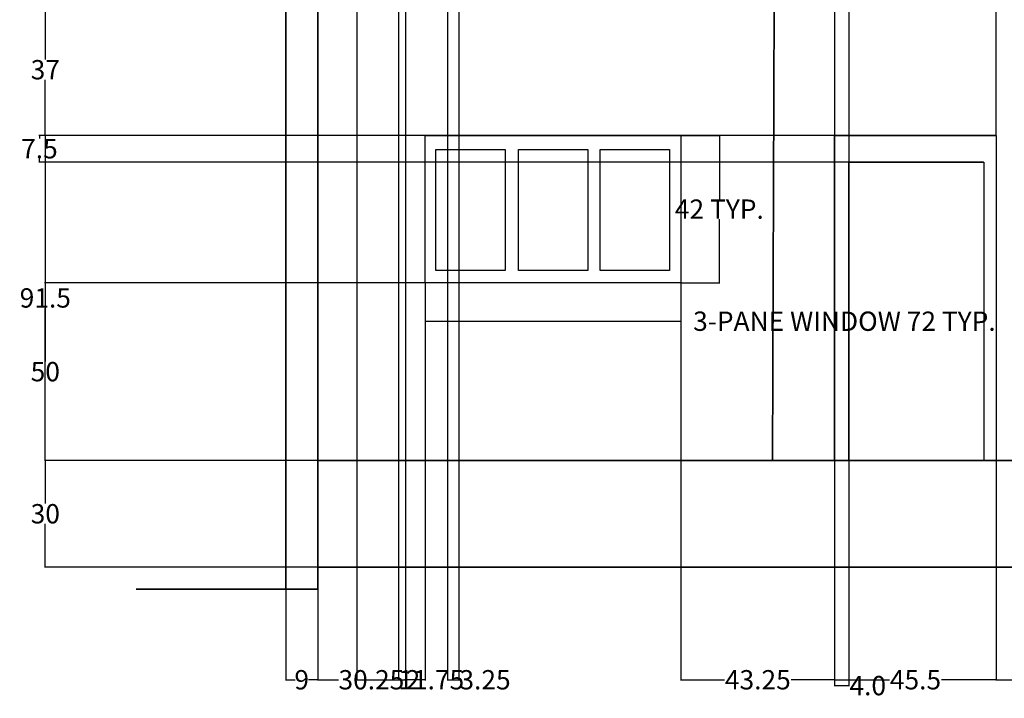
# Model space of a CAD drawing. Units: inches. Extents: x 12 to 590, y 127 to 569.
# Tile 1 of 4: x 17 to 294, y 127 to 318. Entities that reach past the tile are written whole.
import ezdxf

# ---------------------------------------------------------------- set-up
doc = ezdxf.new("R2010")
doc.units = ezdxf.units.IN
doc.header["$MEASUREMENT"] = 0
for name, color, linetype, lineweight in [('A-ANNO-DIMS', 2, 'Continuous', 18), ('A-DOOR', 3, 'Continuous', 25), ('A-ELEV', 7, 'Continuous', 35), ('A-GLAZ', 4, 'Continuous', 25)]:
    doc.layers.add(name, color=color, linetype=linetype, lineweight=lineweight)
doc.styles.get("Standard").update_dxf_attribs({"font": 'arial.ttf'})
doc.dimstyles.get("Standard").update_dxf_attribs({"dimtxt": 5.4375, "dimasz": 0.18, "dimexe": 0.18, "dimexo": 0.0625, "dimgap": 0.09, "dimtad": 0, "dimtih": 1, "dimtoh": 1, "dimdec": 4, "dimzin": 0, "dimdsep": 46, "dimlunit": 4, "dimtxsty": 'Standard', "dimcen": 0.09, "dimadec": 0, "dimazin": 0, "dimtfac": 1, "dimtdec": 4, "dimtofl": 0, "dimtmove": 0, "dimatfit": 3, "dimfxl": 1, "dimtolj": 1, "dimtzin": 0, "dimarcsym": 0})

# ---------------------------------------------------------------- blocks, each defined once
blk = doc.blocks.new('WIN-3PANE')
for points in [[(0, 41.5), (72, 41.5), (72, 0), (0, 0)], [(3, 37.5), (22.5, 37.5), (22.5, 3.5), (3, 3.5)], [(26.25, 37.5), (45.75, 37.5), (45.75, 3.5), (26.25, 3.5)], [(49.25, 37.5), (68.75, 37.5), (68.75, 3.5), (49.25, 3.5)]]:
    blk.add_lwpolyline(points, close=True)
blk = doc.blocks.new('*D3')
at = {"layer": 'A-ANNO-DIMS', "color": 0, "lineweight": -2, "transparency": 16777216}
for p, q in [((130.75, 243.44), (130.75, 232.52)), ((202.75, 243.44), (202.75, 232.52)), ((130.93, 232.7), (202.57, 232.7)), ((202.75, 232.7), (202.93, 232.7))]:
    blk.add_line(p, q, dxfattribs=at)
at = {"layer": 'A-ANNO-DIMS', "color": 0, "transparency": 16777216}
for points in [[(130.93, 232.73), (130.93, 232.67), (130.75, 232.7)], [(202.57, 232.73), (202.57, 232.67), (202.75, 232.7)]]:
    blk.add_solid(points, dxfattribs=at)
at = {"layer": 'Defpoints', "color": 0, "transparency": 16777216}
for p in [(130.75, 243.5), (202.75, 243.5), (202.75, 232.7)]:
    blk.add_point(p, dxfattribs=at)
at = {"layer": 'A-ANNO-DIMS', "color": 0, "transparency": 16777216, "insert": (248.75, 232.7), "char_height": 5.4375, "attachment_point": 5}
blk.add_mtext('\\A1;3-PANE WINDOW 72 TYP.', dxfattribs=at)
blk = doc.blocks.new('*D4')
at = {"layer": 'A-ANNO-DIMS', "color": 0, "lineweight": -2, "transparency": 16777216}
for p, q in [((202.81, 285), (213.73, 285)), ((213.55, 284.82), (213.55, 267.07)), ((213.55, 243.68), (213.55, 261.43)), ((202.81, 243.5), (213.73, 243.5))]:
    blk.add_line(p, q, dxfattribs=at)
at = {"layer": 'A-ANNO-DIMS', "color": 0, "transparency": 16777216}
for points in [[(213.52, 284.82), (213.58, 284.82), (213.55, 285)], [(213.52, 243.68), (213.58, 243.68), (213.55, 243.5)]]:
    blk.add_solid(points, dxfattribs=at)
at = {"layer": 'Defpoints', "color": 0, "transparency": 16777216}
for p in [(202.75, 285), (213.55, 285), (202.75, 243.5)]:
    blk.add_point(p, dxfattribs=at)
at = {"layer": 'A-ANNO-DIMS', "color": 0, "transparency": 16777216, "insert": (213.55, 264.25), "char_height": 5.4375, "attachment_point": 5}
blk.add_mtext('\\A1;42 TYP.', dxfattribs=at)
blk = doc.blocks.new('*D16')
at = {"layer": 'A-ANNO-DIMS', "color": 0, "lineweight": -2, "transparency": 16777216}
for p, q in [((100.44, 193.5), (23.66, 193.5)), ((23.84, 193.32), (23.84, 181.37)), ((23.84, 163.68), (23.84, 175.63)), ((100.44, 163.5), (23.66, 163.5))]:
    blk.add_line(p, q, dxfattribs=at)
at = {"layer": 'A-ANNO-DIMS', "color": 0, "transparency": 16777216}
for points in [[(23.81, 193.32), (23.87, 193.32), (23.84, 193.5)], [(23.81, 163.68), (23.87, 163.68), (23.84, 163.5)]]:
    blk.add_solid(points, dxfattribs=at)
at = {"layer": 'Defpoints', "color": 0, "transparency": 16777216}
for p in [(23.84, 193.5), (100.5, 193.5), (100.5, 163.5)]:
    blk.add_point(p, dxfattribs=at)
at = {"layer": 'A-ANNO-DIMS', "color": 0, "transparency": 16777216, "insert": (23.84, 178.5), "char_height": 5.438, "attachment_point": 5}
blk.add_mtext('\\A1;30', dxfattribs=at)
blk = doc.blocks.new('*D20')
at = {"layer": 'A-ANNO-DIMS', "color": 0, "lineweight": -2, "transparency": 16777216}
for p, q in [((100.5, 163.44), (100.5, 131.59)), ((91.5, 157.25), (91.5, 131.59)), ((91.68, 131.77), (94.12, 131.77)), ((100.32, 131.77), (97.88, 131.77))]:
    blk.add_line(p, q, dxfattribs=at)
at = {"layer": 'A-ANNO-DIMS', "color": 0, "transparency": 16777216}
for points in [[(91.68, 131.8), (91.68, 131.74), (91.5, 131.77)], [(100.32, 131.8), (100.32, 131.74), (100.5, 131.77)]]:
    blk.add_solid(points, dxfattribs=at)
at = {"layer": 'Defpoints', "color": 0, "transparency": 16777216}
for p in [(100.5, 163.5), (91.5, 157.32), (100.5, 131.77)]:
    blk.add_point(p, dxfattribs=at)
at = {"layer": 'A-ANNO-DIMS', "color": 0, "transparency": 16777216, "insert": (96, 131.77), "char_height": 5.438, "attachment_point": 5}
blk.add_mtext('\\A1;9', dxfattribs=at)
blk = doc.blocks.new('*D21')
at = {"layer": 'A-ANNO-DIMS', "color": 0, "lineweight": -2, "transparency": 16777216}
for p, q in [((130.75, 243.44), (130.75, 131.59)), ((100.5, 193.44), (100.5, 131.59)), ((100.68, 131.77), (106.34, 131.77)), ((130.57, 131.77), (124.91, 131.77))]:
    blk.add_line(p, q, dxfattribs=at)
at = {"layer": 'A-ANNO-DIMS', "color": 0, "transparency": 16777216}
for points in [[(100.68, 131.8), (100.68, 131.74), (100.5, 131.77)], [(130.57, 131.8), (130.57, 131.74), (130.75, 131.77)]]:
    blk.add_solid(points, dxfattribs=at)
at = {"layer": 'Defpoints', "color": 0, "transparency": 16777216}
for p in [(130.75, 243.5), (100.5, 193.5), (130.75, 131.77)]:
    blk.add_point(p, dxfattribs=at)
at = {"layer": 'A-ANNO-DIMS', "color": 0, "transparency": 16777216, "insert": (115.62, 131.77), "char_height": 5.438, "attachment_point": 5}
blk.add_mtext('\\A1;30.25', dxfattribs=at)
blk = doc.blocks.new('*D22')
at = {"layer": 'A-ANNO-DIMS', "color": 0, "lineweight": -2, "transparency": 16777216}
for p, q in [((202.75, 243.44), (202.75, 131.59)), ((246, 193.44), (246, 131.59)), ((202.93, 131.77), (214.98, 131.77)), ((245.82, 131.77), (233.77, 131.77))]:
    blk.add_line(p, q, dxfattribs=at)
at = {"layer": 'A-ANNO-DIMS', "color": 0, "transparency": 16777216}
for points in [[(202.93, 131.8), (202.93, 131.74), (202.75, 131.77)], [(245.82, 131.8), (245.82, 131.74), (246, 131.77)]]:
    blk.add_solid(points, dxfattribs=at)
at = {"layer": 'Defpoints', "color": 0, "transparency": 16777216}
for p in [(202.75, 243.5), (246, 193.5), (246, 131.77)]:
    blk.add_point(p, dxfattribs=at)
at = {"layer": 'A-ANNO-DIMS', "color": 0, "transparency": 16777216, "insert": (224.38, 131.77), "char_height": 5.438, "attachment_point": 5}
blk.add_mtext('\\A1;43.25', dxfattribs=at)
blk = doc.blocks.new('*D23')
at = {"layer": 'A-ANNO-DIMS', "color": 0, "lineweight": -2, "transparency": 16777216}
for p, q in [((246, 193.44), (246, 131.59)), ((291.5, 193.44), (291.5, 131.59)), ((246.18, 131.77), (261.47, 131.77)), ((291.32, 131.77), (276.03, 131.77))]:
    blk.add_line(p, q, dxfattribs=at)
at = {"layer": 'A-ANNO-DIMS', "color": 0, "transparency": 16777216}
for points in [[(246.18, 131.8), (246.18, 131.74), (246, 131.77)], [(291.32, 131.8), (291.32, 131.74), (291.5, 131.77)]]:
    blk.add_solid(points, dxfattribs=at)
at = {"layer": 'Defpoints', "color": 0, "transparency": 16777216}
for p in [(246, 193.5), (291.5, 193.5), (291.5, 131.77)]:
    blk.add_point(p, dxfattribs=at)
at = {"layer": 'A-ANNO-DIMS', "color": 0, "transparency": 16777216, "insert": (268.75, 131.77), "char_height": 5.438, "attachment_point": 5}
blk.add_mtext('\\A1;45.5', dxfattribs=at)
blk = doc.blocks.new('*D24')
at = {"layer": 'A-ANNO-DIMS', "color": 0, "lineweight": -2, "transparency": 16777216}
for p, q in [((291.5, 193.44), (291.5, 131.59)), ((310.5, 193.44), (310.5, 131.59)), ((291.68, 131.77), (297.27, 131.77)), ((310.32, 131.77), (304.73, 131.77))]:
    blk.add_line(p, q, dxfattribs=at)
at = {"layer": 'A-ANNO-DIMS', "color": 0, "transparency": 16777216}
for points in [[(291.68, 131.8), (291.68, 131.74), (291.5, 131.77)], [(310.32, 131.8), (310.32, 131.74), (310.5, 131.77)]]:
    blk.add_solid(points, dxfattribs=at)
at = {"layer": 'Defpoints', "color": 0, "transparency": 16777216}
for p in [(291.5, 193.5), (310.5, 193.5), (310.5, 131.77)]:
    blk.add_point(p, dxfattribs=at)
at = {"layer": 'A-ANNO-DIMS', "color": 0, "transparency": 16777216, "insert": (301, 131.77), "char_height": 5.438, "attachment_point": 5}
blk.add_mtext('\\A1;19', dxfattribs=at)
blk = doc.blocks.new('*D29')
at = {"layer": 'A-ANNO-DIMS', "color": 0, "lineweight": -2, "transparency": 16777216}
for p, q in [((130.69, 243.5), (23.66, 243.5)), ((23.84, 243.32), (23.84, 221.37)), ((23.84, 193.68), (23.84, 215.63)), ((100.44, 193.5), (23.66, 193.5))]:
    blk.add_line(p, q, dxfattribs=at)
at = {"layer": 'A-ANNO-DIMS', "color": 0, "transparency": 16777216}
for points in [[(23.81, 243.32), (23.87, 243.32), (23.84, 243.5)], [(23.81, 193.68), (23.87, 193.68), (23.84, 193.5)]]:
    blk.add_solid(points, dxfattribs=at)
at = {"layer": 'Defpoints', "color": 0, "transparency": 16777216}
for p in [(23.84, 243.5), (130.75, 243.5), (100.5, 193.5)]:
    blk.add_point(p, dxfattribs=at)
at = {"layer": 'A-ANNO-DIMS', "color": 0, "transparency": 16777216, "insert": (23.84, 218.5), "char_height": 5.438, "attachment_point": 5}
blk.add_mtext('\\A1;50', dxfattribs=at)
blk = doc.blocks.new('*D30')
at = {"layer": 'A-ANNO-DIMS', "color": 0, "lineweight": -2, "transparency": 16777216}
for p, q in [((100.44, 322), (23.66, 322)), ((23.84, 321.82), (23.84, 306.37)), ((23.84, 285.18), (23.84, 300.63)), ((130.69, 285), (23.66, 285))]:
    blk.add_line(p, q, dxfattribs=at)
at = {"layer": 'A-ANNO-DIMS', "color": 0, "transparency": 16777216}
for points in [[(23.81, 321.82), (23.87, 321.82), (23.84, 322)], [(23.81, 285.18), (23.87, 285.18), (23.84, 285)]]:
    blk.add_solid(points, dxfattribs=at)
at = {"layer": 'Defpoints', "color": 0, "transparency": 16777216}
for p in [(23.84, 322), (100.5, 322), (130.75, 285)]:
    blk.add_point(p, dxfattribs=at)
at = {"layer": 'A-ANNO-DIMS', "color": 0, "transparency": 16777216, "insert": (23.84, 303.5), "char_height": 5.438, "attachment_point": 5}
blk.add_mtext('\\A1;37', dxfattribs=at)
blk = doc.blocks.new('*D31')
at = {"layer": 'A-ANNO-DIMS', "color": 0, "lineweight": -2, "transparency": 16777216}
for p, q in [((245.94, 285), (23.66, 285)), ((23.84, 284.82), (23.84, 242.12)), ((23.84, 193.68), (23.84, 236.38)), ((245.94, 193.5), (23.66, 193.5))]:
    blk.add_line(p, q, dxfattribs=at)
at = {"layer": 'A-ANNO-DIMS', "color": 0, "transparency": 16777216}
for points in [[(23.81, 284.82), (23.87, 284.82), (23.84, 285)], [(23.81, 193.68), (23.87, 193.68), (23.84, 193.5)]]:
    blk.add_solid(points, dxfattribs=at)
at = {"layer": 'Defpoints', "color": 0, "transparency": 16777216}
for p in [(23.84, 285), (246, 285), (246, 193.5)]:
    blk.add_point(p, dxfattribs=at)
at = {"layer": 'A-ANNO-DIMS', "color": 0, "transparency": 16777216, "insert": (23.84, 239.25), "char_height": 5.438, "attachment_point": 5}
blk.add_mtext('\\A1;91.5', dxfattribs=at)
blk = doc.blocks.new('*D44')
at = {"layer": 'A-ANNO-DIMS', "color": 0, "lineweight": -2, "transparency": 16777216}
for p, q in [((111.5, 347.94), (111.5, 131.59)), ((123.25, 347.94), (123.25, 131.59)), ((111.68, 131.77), (123.07, 131.77)), ((123.25, 131.77), (123.43, 131.77))]:
    blk.add_line(p, q, dxfattribs=at)
at = {"layer": 'A-ANNO-DIMS', "color": 0, "transparency": 16777216}
for points in [[(111.68, 131.8), (111.68, 131.74), (111.5, 131.77)], [(123.07, 131.8), (123.07, 131.74), (123.25, 131.77)]]:
    blk.add_solid(points, dxfattribs=at)
at = {"layer": 'Defpoints', "color": 0, "transparency": 16777216}
for p in [(111.5, 348), (123.25, 348), (123.25, 131.77)]:
    blk.add_point(p, dxfattribs=at)
at = {"layer": 'A-ANNO-DIMS', "color": 0, "transparency": 16777216, "insert": (132.46, 131.77), "char_height": 5.438, "attachment_point": 5}
blk.add_mtext('\\A1;11.75', dxfattribs=at)
blk = doc.blocks.new('*D45')
at = {"layer": 'A-ANNO-DIMS', "color": 0, "lineweight": -2, "transparency": 16777216}
for p, q in [((123.25, 347.94), (123.25, 131.59)), ((125.25, 347.94), (125.25, 131.59)), ((123.43, 131.77), (125.07, 131.77)), ((125.25, 131.77), (125.43, 131.77))]:
    blk.add_line(p, q, dxfattribs=at)
at = {"layer": 'A-ANNO-DIMS', "color": 0, "transparency": 16777216}
for points in [[(123.43, 131.8), (123.43, 131.74), (123.25, 131.77)], [(125.07, 131.8), (125.07, 131.74), (125.25, 131.77)]]:
    blk.add_solid(points, dxfattribs=at)
at = {"layer": 'Defpoints', "color": 0, "transparency": 16777216}
for p in [(123.25, 348), (125.25, 348), (125.25, 131.77)]:
    blk.add_point(p, dxfattribs=at)
at = {"layer": 'A-ANNO-DIMS', "color": 0, "transparency": 16777216, "insert": (127.32, 131.77), "char_height": 5.438, "attachment_point": 5}
blk.add_mtext('\\A1;2', dxfattribs=at)
blk = doc.blocks.new('*D46')
at = {"layer": 'A-ANNO-DIMS', "color": 0, "lineweight": -2, "transparency": 16777216}
for p, q in [((137, 347.94), (137, 131.59)), ((140.25, 347.94), (140.25, 131.59)), ((137.18, 131.77), (140.07, 131.77)), ((140.25, 131.77), (140.43, 131.77))]:
    blk.add_line(p, q, dxfattribs=at)
at = {"layer": 'A-ANNO-DIMS', "color": 0, "transparency": 16777216}
for points in [[(137.18, 131.8), (137.18, 131.74), (137, 131.77)], [(140.07, 131.8), (140.07, 131.74), (140.25, 131.77)]]:
    blk.add_solid(points, dxfattribs=at)
at = {"layer": 'Defpoints', "color": 0, "transparency": 16777216}
for p in [(137, 348), (140.25, 348), (140.25, 131.77)]:
    blk.add_point(p, dxfattribs=at)
at = {"layer": 'A-ANNO-DIMS', "color": 0, "transparency": 16777216, "insert": (147.6, 131.77), "char_height": 5.438, "attachment_point": 5}
blk.add_mtext('\\A1;3.25', dxfattribs=at)
blk = doc.blocks.new('*D56')
at = {"layer": 'A-ANNO-DIMS', "color": 0, "lineweight": -2, "transparency": 16777216}
for p, q in [((246, 284.94), (246, 129.94)), ((250, 277.44), (250, 129.94)), ((246.18, 130.12), (249.82, 130.12)), ((250, 130.12), (250.18, 130.12))]:
    blk.add_line(p, q, dxfattribs=at)
at = {"layer": 'A-ANNO-DIMS', "color": 0, "transparency": 16777216}
for points in [[(246.18, 130.15), (246.18, 130.09), (246, 130.12)], [(249.82, 130.15), (249.82, 130.09), (250, 130.12)]]:
    blk.add_solid(points, dxfattribs=at)
at = {"layer": 'Defpoints', "color": 0, "transparency": 16777216}
for p in [(246, 285), (250, 277.5), (250, 130.12)]:
    blk.add_point(p, dxfattribs=at)
at = {"layer": 'A-ANNO-DIMS', "color": 0, "transparency": 16777216, "insert": (255.32, 130.12), "char_height": 5.438, "attachment_point": 5}
blk.add_mtext('\\A1;4.0', dxfattribs=at)
blk = doc.blocks.new('*D57')
at = {"layer": 'A-ANNO-DIMS', "color": 0, "lineweight": -2, "transparency": 16777216}
for p, q in [((291.44, 285), (22.01, 285)), ((22.19, 284.82), (22.19, 284.11)), ((287.94, 277.5), (22.01, 277.5)), ((22.19, 277.68), (22.19, 278.39))]:
    blk.add_line(p, q, dxfattribs=at)
at = {"layer": 'A-ANNO-DIMS', "color": 0, "transparency": 16777216}
for points in [[(22.16, 284.82), (22.22, 284.82), (22.19, 285)], [(22.16, 277.68), (22.22, 277.68), (22.19, 277.5)]]:
    blk.add_solid(points, dxfattribs=at)
at = {"layer": 'Defpoints', "color": 0, "transparency": 16777216}
for p in [(291.5, 285), (22.19, 277.5), (288, 277.5)]:
    blk.add_point(p, dxfattribs=at)
at = {"layer": 'A-ANNO-DIMS', "color": 0, "transparency": 16777216, "insert": (22.19, 281.25), "char_height": 5.438, "attachment_point": 5}
blk.add_mtext('\\A1;7.5', dxfattribs=at)
blk = doc.blocks.new('*D58')
at = {"layer": 'A-ANNO-DIMS', "color": 0, "lineweight": -2, "transparency": 16777216}
for p, q in [((246, 428.94), (246, 129.94)), ((250, 424.94), (250, 129.94)), ((246.18, 130.12), (249.82, 130.12)), ((250, 130.12), (250.18, 130.12))]:
    blk.add_line(p, q, dxfattribs=at)
at = {"layer": 'A-ANNO-DIMS', "color": 0, "transparency": 16777216}
for points in [[(246.18, 130.15), (246.18, 130.09), (246, 130.12)], [(249.82, 130.15), (249.82, 130.09), (250, 130.12)]]:
    blk.add_solid(points, dxfattribs=at)
at = {"layer": 'Defpoints', "color": 0, "transparency": 16777216}
for p in [(246, 429), (250, 425), (250, 130.12)]:
    blk.add_point(p, dxfattribs=at)
at = {"layer": 'A-ANNO-DIMS', "color": 0, "transparency": 16777216, "insert": (255.32, 130.12), "char_height": 5.438, "attachment_point": 5}
blk.add_mtext('\\A1;4.0', dxfattribs=at)
blk = doc.blocks.new('*D60')
at = {"layer": 'A-ANNO-DIMS', "color": 0, "lineweight": -2, "transparency": 16777216}
for p, q in [((291.5, 285.06), (291.5, 565.38)), ((350.5, 285.06), (350.5, 565.38)), ((291.68, 565.2), (313.86, 565.2)), ((350.32, 565.2), (328.14, 565.2))]:
    blk.add_line(p, q, dxfattribs=at)
at = {"layer": 'A-ANNO-DIMS', "color": 0, "transparency": 16777216}
for points in [[(291.68, 565.23), (291.68, 565.17), (291.5, 565.2)], [(350.32, 565.23), (350.32, 565.17), (350.5, 565.2)]]:
    blk.add_solid(points, dxfattribs=at)
at = {"layer": 'Defpoints', "color": 0, "transparency": 16777216}
for p in [(350.5, 565.2), (291.5, 285), (350.5, 285)]:
    blk.add_point(p, dxfattribs=at)
at = {"layer": 'A-ANNO-DIMS', "color": 0, "transparency": 16777216, "insert": (321, 565.2), "char_height": 5.438, "attachment_point": 5}
blk.add_mtext('\\A1;59.0', dxfattribs=at)

msp = doc.modelspace()

# ---------------------------------------------------------------- linework, layer by layer
at = {"layer": 'A-DOOR'}
for points in [[(246, 285), (291.5, 285), (291.5, 193.5), (246, 193.5)], [(250, 277.5), (288, 277.5), (288, 193.5), (250, 193.5)]]:
    msp.add_lwpolyline(points, close=True, dxfattribs=at)
at = {"layer": 'A-ELEV'}
for p, q in [((91.5, 301.3163), (91.5, 492)), ((100.5, 301.3163), (100.5, 322)), ((229, 322), (228.5, 193.5)), ((91.5, 231.5), (91.5, 301.3163)), ((100.5, 157.3163), (100.5, 301.3163)), ((91.5, 200.5), (91.5, 231.5)), ((91.5, 200.5), (91.5, 157.3163)), ((100.5, 163.5), (100.5, 193.5)), ((100.5, 193.5), (328.5, 193.5)), ((100.5, 163.5), (422, 163.5)), ((49.391, 157.3163), (100.5, 157.3163))]:
    msp.add_line(p, q, dxfattribs=at)

# ---------------------------------------------------------------- block references
at = {"layer": 'A-GLAZ'}
msp.add_blockref('WIN-3PANE', (130.75, 243.5), dxfattribs=at)

# ---------------------------------------------------------------- dimensions: what is measured, and where the dimension line sits
at = {"layer": 'A-ANNO-DIMS'}
for base, p1, p2, override, picture, middle in [((350.5, 565.2), (291.5, 285), (350.5, 285), {"dimdec": 1, "dimlfac": 1, "dimrnd": 0, "dimzin": 0, "dimdsep": 46, "dimlunit": 2}, '*D60', (321, 565.2)), ((250, 130.1163), (246, 429), (250, 425), {"dimdec": 1, "dimlfac": 1, "dimrnd": 0, "dimzin": 0, "dimdsep": 46, "dimlunit": 2}, '*D58', (255.3199, 130.1163)), ((123.25, 131.7663), (111.5, 348), (123.25, 348), {"dimdec": 2, "dimlfac": 1, "dimrnd": 0, "dimzin": 0, "dimdsep": 46, "dimlunit": 2}, '*D44', (132.4589, 131.7663)), ((125.25, 131.7663), (123.25, 348), (125.25, 348), {"dimdec": 0, "dimlfac": 1, "dimrnd": 0, "dimzin": 0, "dimdsep": 46, "dimlunit": 2}, '*D45', (127.3208, 131.7663)), ((140.25, 131.7663), (137, 348), (140.25, 348), {"dimdec": 2, "dimlfac": 1, "dimrnd": 0, "dimzin": 0, "dimdsep": 46, "dimlunit": 2}, '*D46', (147.6006, 131.7663)), ((250, 130.1163), (246, 285), (250, 277.5), {"dimdec": 1, "dimlfac": 1, "dimrnd": 0, "dimzin": 0, "dimdsep": 46, "dimlunit": 2}, '*D56', (255.3199, 130.1163)), ((130.75, 131.7663), (100.5, 193.5), (130.75, 243.5), {"dimdec": 2, "dimlfac": 1, "dimrnd": 0, "dimzin": 0, "dimdsep": 46, "dimlunit": 2}, '*D21', (115.625, 131.7663)), ((246, 131.7663), (202.75, 243.5), (246, 193.5), {"dimdec": 2, "dimlfac": 1, "dimrnd": 0, "dimzin": 0, "dimdsep": 46, "dimlunit": 2}, '*D22', (224.375, 131.7663)), ((291.5, 131.7663), (246, 193.5), (291.5, 193.5), {"dimdec": 1, "dimlfac": 1, "dimrnd": 0, "dimzin": 0, "dimdsep": 46, "dimlunit": 2}, '*D23', (268.75, 131.7663)), ((310.5, 131.7663), (291.5, 193.5), (310.5, 193.5), {"dimdec": 0, "dimlfac": 1, "dimrnd": 0, "dimzin": 0, "dimdsep": 46, "dimlunit": 2}, '*D24', (301, 131.7663)), ((100.5, 131.7663), (91.5, 157.3163), (100.5, 163.5), {"dimdec": 0, "dimlfac": 1, "dimrnd": 0, "dimzin": 0, "dimdsep": 46, "dimlunit": 2}, '*D20', (96, 131.7663))]:
    dim = msp.add_linear_dim(base=base, p1=p1, p2=p2, dimstyle='Standard', override=override, dxfattribs=at)
    dim.commit()
    dim.dimension.update_dxf_attribs({"geometry": picture, "text_midpoint": middle})
for base, p1, p2, override, picture, middle in [((23.841, 322), (130.75, 285), (100.5, 322), {"dimdec": 0, "dimlfac": 1, "dimrnd": 0, "dimzin": 0, "dimdsep": 46, "dimlunit": 2}, '*D30', (23.841, 303.5)), ((23.841, 285), (246, 193.5), (246, 285), {"dimdec": 1, "dimlfac": 1, "dimrnd": 0, "dimzin": 0, "dimdsep": 46, "dimlunit": 2}, '*D31', (23.841, 239.25)), ((22.191, 277.5), (291.5, 285), (288, 277.5), {"dimdec": 1, "dimlfac": 1, "dimrnd": 0, "dimzin": 0, "dimdsep": 46, "dimlunit": 2}, '*D57', (22.191, 281.25)), ((23.841, 243.5), (100.5, 193.5), (130.75, 243.5), {"dimdec": 0, "dimlfac": 1, "dimrnd": 0, "dimzin": 0, "dimdsep": 46, "dimlunit": 2}, '*D29', (23.841, 218.5)), ((23.841, 193.5), (100.5, 163.5), (100.5, 193.5), {"dimdec": 0, "dimlfac": 1, "dimrnd": 0, "dimzin": 0, "dimdsep": 46, "dimlunit": 2}, '*D16', (23.841, 178.5))]:
    dim = msp.add_linear_dim(base=base, p1=p1, p2=p2, angle=90, dimstyle='Standard', override=override, dxfattribs=at)
    dim.commit()
    dim.dimension.update_dxf_attribs({"geometry": picture, "text_midpoint": middle})
dim = msp.add_linear_dim(base=(213.55, 285), p1=(202.75, 243.5), p2=(202.75, 285), angle=90, text='<> TYP.', dimstyle='Standard', override={"dimdec": 0, "dimlfac": 1, "dimrnd": 0, "dimzin": 0, "dimdsep": 46, "dimlunit": 2}, dxfattribs=at)
dim.commit()
dim.dimension.update_dxf_attribs({"geometry": '*D4', "text_midpoint": (213.55, 264.25)})
dim = msp.add_linear_dim(base=(202.75, 232.7), p1=(130.75, 243.5), p2=(202.75, 243.5), text='3-PANE WINDOW <> TYP.', dimstyle='Standard', override={"dimdec": 0, "dimlfac": 1, "dimrnd": 0, "dimzin": 0, "dimdsep": 46, "dimlunit": 2}, dxfattribs=at)
dim.commit()
dim.dimension.update_dxf_attribs({"geometry": '*D3', "text_midpoint": (248.7473, 232.7)})

doc.saveas('drawing.dxf')
